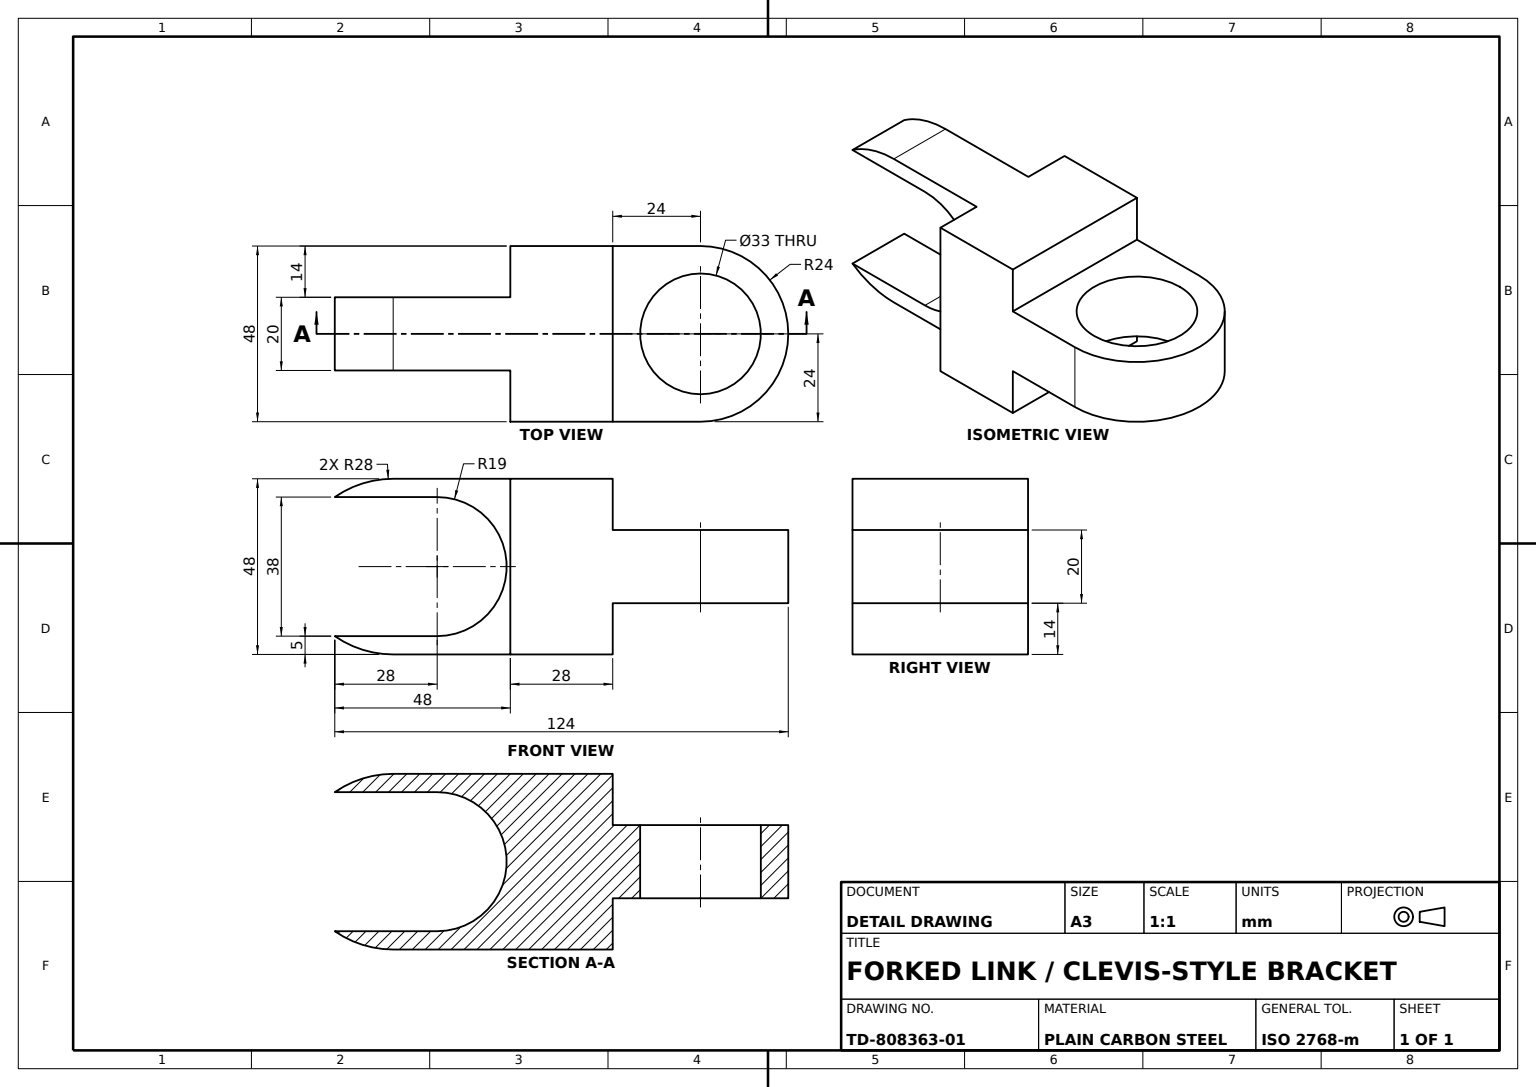
from build123d import *

# Parameters (mm, degrees)
BASE_BLOCK_SKETCH_W       = 28
BASE_BLOCK_SKETCH_H       = 48
BASE_BLOCK_DEPTH          = 24
FORK_ARMS_DEPTH           = 10
FORK_ARC_CUT_SKETCH_R33_R = 16.5
FORK_ARC_CUT_DEPTH        = 20
EYE_START                 = -24
EYE_LUG_WITH_BORE_DEPTH   = 10


with BuildPart() as part:
    # Base Block Sketch → Base Block (new, symmetric)
    with BuildSketch(Plane.XY):
        with Locations((14, -24)):
            Rectangle(BASE_BLOCK_SKETCH_W, BASE_BLOCK_SKETCH_H)
    extrude(amount=BASE_BLOCK_DEPTH, both=True)

    # Fork Arms Sketch → Fork Arms (add, symmetric)
    with BuildSketch(Plane(origin=(0, -24, 0), x_dir=(1, 0, 0), z_dir=(0, 1, 0))):
        with BuildLine():
            Line((52, 24), (28, 24))
            Line((28, 24), (28, -24))
            Line((28, -24), (52, -24))
            ThreePointArc((52, -24), (76, 0), (52, 24))
        make_face()
    extrude(amount=FORK_ARMS_DEPTH, both=True)

    # Fork Arc Cut Sketch R33 → Fork Arc Cut (cut)
    with BuildSketch(Plane(origin=(0, -14, 0), x_dir=(1, 0, 0), z_dir=(0, 1, 0))):
        with Locations(Location((52, 0, 0), (0, 0, 270))):
            Circle(FORK_ARC_CUT_SKETCH_R33_R)
    extrude(amount=-FORK_ARC_CUT_DEPTH, mode=Mode.SUBTRACT)

    # Eye Lug Sketch → Eye Lug With Bore (add, symmetric)
    with BuildSketch(Plane.XY.offset(24).offset(EYE_START)):
        with BuildLine():
            Line((0, 0), (-32.031280577, 0))
            ThreePointArc((-32.031280577, 0), (-40.397880843, -1.279221568), (-48, -5))
            Line((-48, -5), (-20, -5))
            ThreePointArc((-20, -5), (-1, -24), (-20, -43))
            Line((-20, -43), (-48, -43))
            ThreePointArc((-48, -43), (-40.397880843, -46.720778432), (-32.031280577, -48))
            Line((-32.031280577, -48), (0, -48))
            Line((0, -48), (0, 0))
        make_face()
    extrude(amount=EYE_LUG_WITH_BORE_DEPTH, both=True)


solid = part.part
